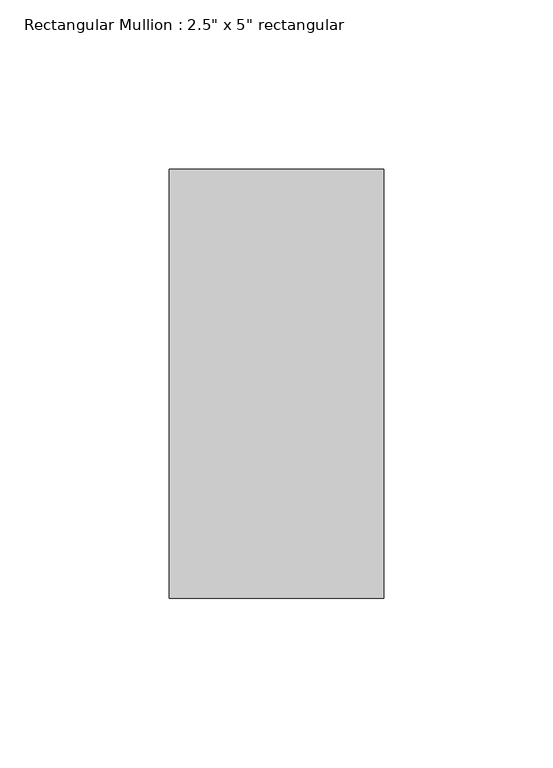
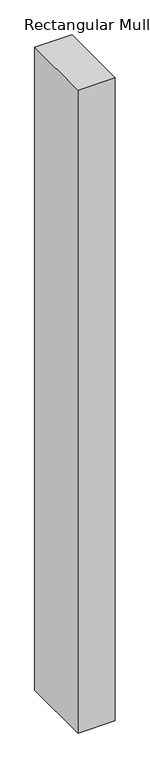
"""IFC4 building model written with IfcOpenShell, lengths in millimetres: member geometry."""

from ifc_helpers import new_model, si_unit, frame, origin, place, context, project, spatial, polyline, outline, extrude, source, transform, mapped, element, save


def member_1e0ac351(model_context):
    return source(origin(), model_context, "Body", "SweptSolid", [
        extrude(outline(polyline([(0.0, 63.5), (0.0, -63.5), (-63.5, -63.5), (-63.5, 63.5), (0.0, 63.5)])), frame((0.0, 0.0, -1155.3877959), z_axis=(0.0, 0.0, 1.0), x_axis=(1.0, 0.0, 0.0)), (0.0, 0.0, 1.0), 1155.3877959),
    ])


if __name__ == "__main__":
    model = new_model("IFC4")
    model_context = context("Model", 3, world=origin())
    ifc_project = project(units=[si_unit("LENGTHUNIT", "METRE", prefix="MILLI")], contexts=[model_context])
    site = spatial("IfcSite", under=ifc_project)
    building = spatial("IfcBuilding", under=site)
    placement = place(None, origin())
    member_shape = member_1e0ac351(model_context)
    element("IfcMember", 1, ObjectType="Rectangular Mullion : 2.5\" x 5\" rectangular", at=placement, inside=building, context=model_context, shape_type="MappedRepresentation", body=[
        mapped(member_shape, transform((0.0, 0.0, 0.0), x_axis=(1.0, 0.0, 0.0), y_axis=(0.0, 1.0, 0.0), z_axis=(0.0, 0.0, 1.0))),
    ])
    save(model, "model.ifc")

# Revit data of these elements
# Type "Rectangular Mullion : 2.5\" x 5\" rectangular"
#   built-in parameter 1007304 = 0.416667 (stored number, unit not read)
#   built-in parameter 1007301 = 0.104167 (stored number, unit not read)
#   built-in parameter 1007300 = 0.104167 (stored number, unit not read)
# Element 1 (IfcMember, "Rectangular Mullion : 2.5\" x 5\" rectangular")
#   Materials on its faces: "Aluminum"
# Materials
#   "Aluminum": class "Metal", colour RGB 247 247 247, transparency 0, Description = "Aluminum 6061", Cost = 0
